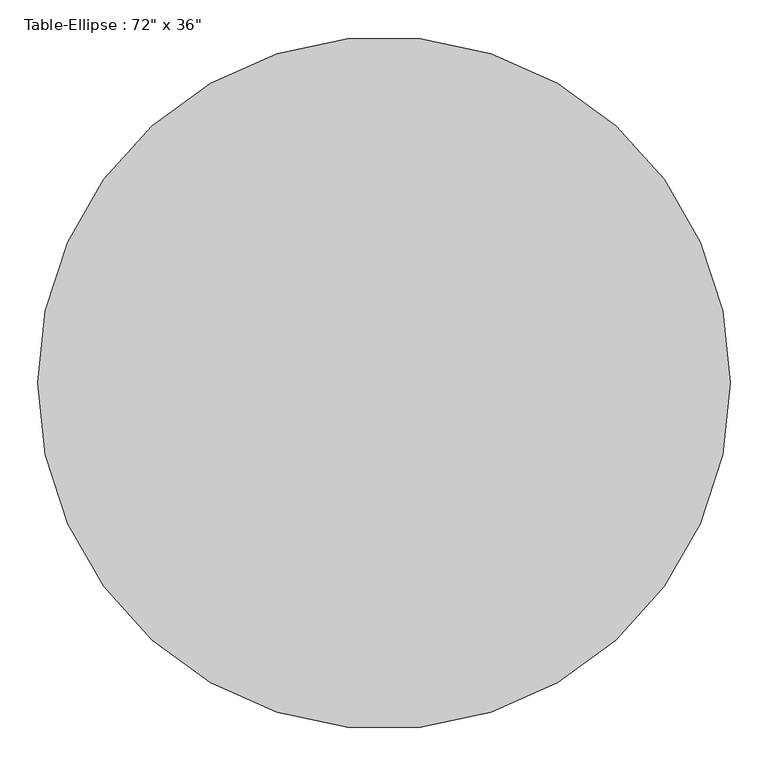
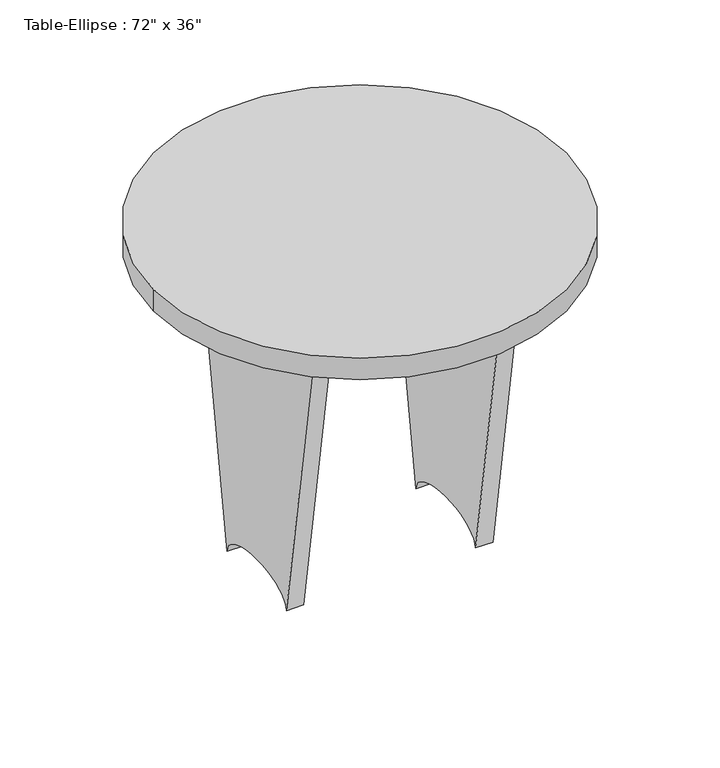
"""IFC4 building model written with IfcOpenShell, lengths in millimetres: furniture geometry."""

from ifc_helpers import new_model, si_unit, point, frame, origin, place, context, project, spatial, circle_curve, ellipse_curve, trimmed, source, transform, mapped, element, save
from ifc_brep_helpers import plane_surface, extruded_surface, advanced_brep


def furniture_4bee3317(model_context):
    return source(origin(), model_context, "Body", "AdvancedBrep", [
        advanced_brep(
        [(-190.5, 19.05, 711.2), (190.5, 19.05, 711.2), (190.5, 19.05, 474.1333333), (-190.5, 19.05, 474.1333333), (-190.5, -19.05, 711.2), (-190.5, -19.05, 474.1333333), (190.5, -19.05, 474.1333333), (190.5, -19.05, 711.2)],
        [
            (0, 1),
            (1, 2),
            (2, 3, ellipse_curve(frame((0.0, 19.05, 474.1333333), z_axis=(0.0, -1.0, 0.0), x_axis=(1.0, 0.0, 0.0)), 190.5, 101.6)),
            (3, 0),
            (4, 5),
            (5, 6, ellipse_curve(frame((0.0, -19.05, 474.1333333), z_axis=(0.0, 1.0, 0.0), x_axis=(1.0, 0.0, 0.0)), 190.5, 101.6)),
            (6, 7),
            (7, 4),
            (0, 4),
            (7, 1),
            (6, 2),
            (5, 3),
        ],
        [
            plane_surface(frame((-190.5, 19.05, 711.2), z_axis=(0.0, 1.0, 0.0), x_axis=(1.0, 0.0, 0.0))),
            plane_surface(frame((-190.5, -19.05, 711.2), z_axis=(0.0, -1.0, 0.0), x_axis=(-1.0, 0.0, 0.0))),
            plane_surface(frame((-190.5, 19.05, 711.2), z_axis=(0.0, 0.0, 1.0), x_axis=(0.0, -1.0, 0.0))),
            plane_surface(frame((190.5, 19.05, 711.2), z_axis=(1.0, 0.0, 0.0), x_axis=(0.0, -1.0, 0.0))),
            extruded_surface(trimmed(ellipse_curve(frame((0.0, -57.15, 474.1333333), z_axis=(0.0, -1.0, 0.0), x_axis=(1.0, 0.0, 0.0)), 190.5, 101.6), [point((190.5, -57.15, 474.1333333))], [point((-190.5, -57.15, 474.1333333))], True, "CARTESIAN"), (0.0, 38.099999999999994, 0.0), 38.099999999999994),
            plane_surface(frame((-190.5, 19.05, 474.1333333), z_axis=(-1.0, 0.0, 0.0), x_axis=(0.0, -1.0, 0.0))),
        ],
        [
            (0, [[1, 2, 3, 4]]),
            (1, [[5, 6, 7, 8]]),
            (2, [[-1, 9, -8, 10]]),
            (3, [[-2, -10, -7, 11]]),
            (4, [[-3, -11, -6, 12]]),
            (5, [[-4, -12, -5, -9]]),
        ],
    ),
        advanced_brep(
        [(228.6, 228.6, 711.2), (228.6, -228.6, 711.2), (228.6, -114.3, 0.0), (228.6, 114.3, 0.0), (190.5, 228.6, 711.2), (190.5, 114.3, 0.0), (190.5, -114.3, 0.0), (190.5, -228.6, 711.2)],
        [
            (0, 1),
            (1, 2),
            (2, 3, ellipse_curve(frame((228.6, 0.0, 0.0), z_axis=(-1.0, 0.0, 0.0), x_axis=(0.0, 1.0, 0.0)), 114.3, 50.8)),
            (3, 0),
            (4, 5),
            (5, 6, ellipse_curve(frame((190.5, 0.0, 0.0), z_axis=(1.0, 0.0, 0.0), x_axis=(0.0, 1.0, 0.0)), 114.3, 50.8)),
            (6, 7),
            (7, 4),
            (0, 4),
            (7, 1),
            (6, 2),
            (5, 3),
        ],
        [
            plane_surface(frame((228.6, -228.6, 711.2), z_axis=(1.0, 0.0, 0.0), x_axis=(0.0, -1.0, 0.0))),
            plane_surface(frame((190.5, -228.6, 711.2), z_axis=(-1.0, 0.0, 0.0), x_axis=(0.0, 1.0, 0.0))),
            plane_surface(frame((228.6, 228.6, 711.2), z_axis=(0.0, 0.0, 1.0), x_axis=(-1.0, 0.0, 0.0))),
            plane_surface(frame((228.6, -228.6, 711.2), z_axis=(0.0, -0.9873303712766982, -0.158678095383759), x_axis=(-1.0, 0.0, 0.0))),
            extruded_surface(trimmed(ellipse_curve(frame((152.4, 0.0, 0.0), z_axis=(-1.0, 0.0, 0.0), x_axis=(0.0, 1.0, 0.0)), 114.3, 50.8), [point((152.4, -114.3, 0.0))], [point((152.4, 114.3, 0.0))], True, "CARTESIAN"), (38.099999999999994, 0.0, 0.0), 38.099999999999994),
            plane_surface(frame((228.6, 114.3, 0.0), z_axis=(0.0, 0.9873303712767002, -0.15867809538374666), x_axis=(-1.0, 0.0, 0.0))),
        ],
        [
            (0, [[1, 2, 3, 4]]),
            (1, [[5, 6, 7, 8]]),
            (2, [[-1, 9, -8, 10]]),
            (3, [[-2, -10, -7, 11]]),
            (4, [[-3, -11, -6, 12]]),
            (5, [[-4, -12, -5, -9]]),
        ],
    ),
        advanced_brep(
        [(-190.5, 228.6, 711.2), (-190.5, -228.6, 711.2), (-190.5, -114.3, 0.0), (-190.5, 114.3, 0.0), (-228.6, 228.6, 711.2), (-228.6, 114.3, 0.0), (-228.6, -114.3, 0.0), (-228.6, -228.6, 711.2)],
        [
            (0, 1),
            (1, 2),
            (2, 3, ellipse_curve(frame((-190.5, 0.0, 0.0), z_axis=(-1.0, 0.0, 0.0), x_axis=(0.0, 1.0, 0.0)), 114.3, 50.8)),
            (3, 0),
            (4, 5),
            (5, 6, ellipse_curve(frame((-228.6, 0.0, 0.0), z_axis=(1.0, 0.0, 0.0), x_axis=(0.0, 1.0, 0.0)), 114.3, 50.8)),
            (6, 7),
            (7, 4),
            (0, 4),
            (7, 1),
            (6, 2),
            (5, 3),
        ],
        [
            plane_surface(frame((-190.5, -228.6, 711.2), z_axis=(1.0, 0.0, 0.0), x_axis=(0.0, -1.0, 0.0))),
            plane_surface(frame((-228.6, -228.6, 711.2), z_axis=(-1.0, 0.0, 0.0), x_axis=(0.0, 1.0, 0.0))),
            plane_surface(frame((-190.5, 228.6, 711.2), z_axis=(0.0, 0.0, 1.0), x_axis=(-1.0, 0.0, 0.0))),
            plane_surface(frame((-190.5, -228.6, 711.2), z_axis=(0.0, -0.9873303712766983, -0.15867809538375854), x_axis=(-1.0, 0.0, 0.0))),
            extruded_surface(trimmed(ellipse_curve(frame((-266.7, 0.0, 0.0), z_axis=(-1.0, 0.0, 0.0), x_axis=(0.0, 1.0, 0.0)), 114.3, 50.8), [point((-266.7, -114.3, 0.0))], [point((-266.7, 114.3, 0.0))], True, "CARTESIAN"), (38.099999999999994, 0.0, 0.0), 38.099999999999994),
            plane_surface(frame((-190.5, 114.3, 0.0), z_axis=(0.0, 0.9873303712766998, -0.15867809538374977), x_axis=(-1.0, 0.0, 0.0))),
        ],
        [
            (0, [[1, 2, 3, 4]]),
            (1, [[5, 6, 7, 8]]),
            (2, [[-1, 9, -8, 10]]),
            (3, [[-2, -10, -7, 11]]),
            (4, [[-3, -11, -6, 12]]),
            (5, [[-4, -12, -5, -9]]),
        ],
    ),
        advanced_brep(
        [(-457.2, 0.0, 762.0), (457.2, 0.0, 762.0), (-457.2, 0.0, 711.2), (457.2, 0.0, 711.2)],
        [
            (0, 1, circle_curve(frame((0.0, 0.0, 762.0), z_axis=(0.0, 0.0, 1.0), x_axis=(1.0, 0.0, 0.0)), 457.2)),
            (1, 0, circle_curve(frame((0.0, 0.0, 762.0), z_axis=(0.0, 0.0, 1.0), x_axis=(1.0, 0.0, 0.0)), 457.2)),
            (2, 3, ellipse_curve(frame((0.0, 0.0, 711.2), z_axis=(0.0, 0.0, -1.0), x_axis=(1.0, 0.0, 0.0)), 457.2, 457.2)),
            (3, 2, ellipse_curve(frame((0.0, 0.0, 711.2), z_axis=(0.0, 0.0, -1.0), x_axis=(1.0, 0.0, 0.0)), 457.2, 457.2)),
            (0, 2),
            (3, 1),
        ],
        [
            plane_surface(frame((457.2, 0.0, 762.0), z_axis=(0.0, 0.0, 1.0), x_axis=(0.0, 1.0, 0.0))),
            plane_surface(frame((457.2, 0.0, 711.2), z_axis=(0.0, 0.0, -1.0), x_axis=(0.0, -1.0, 0.0))),
            extruded_surface(trimmed(ellipse_curve(frame((0.0, 0.0, 660.4), z_axis=(0.0, 0.0, 1.0), x_axis=(1.0, 0.0, 0.0)), 457.2, 457.2), [point((-457.2, 0.0, 660.4))], [point((457.2, 0.0, 660.4))], True, "CARTESIAN"), (0.0, 0.0, 50.80000000000007), 50.80000000000007),
            extruded_surface(trimmed(ellipse_curve(frame((0.0, 0.0, 660.4), z_axis=(0.0, 0.0, 1.0), x_axis=(1.0, 0.0, 0.0)), 457.2, 457.2), [point((457.2, 0.0, 660.4))], [point((-457.2, 0.0, 660.4))], True, "CARTESIAN"), (0.0, 0.0, 50.80000000000007), 50.80000000000007),
        ],
        [
            (0, [[1, 2]]),
            (1, [[3, 4]]),
            (2, [[-1, 5, -4, 6]]),
            (3, [[-2, -6, -3, -5]]),
        ],
    ),
    ])


if __name__ == "__main__":
    model = new_model("IFC4")
    model_context = context("Model", 3, world=origin())
    ifc_project = project(units=[si_unit("LENGTHUNIT", "METRE", prefix="MILLI")], contexts=[model_context])
    site = spatial("IfcSite", under=ifc_project)
    building = spatial("IfcBuilding", under=site)
    placement = place(None, origin())
    furniture_shape = furniture_4bee3317(model_context)
    element("IfcFurniture", 1, ObjectType="Table-Ellipse : 72\" x 36\"", at=placement, inside=building, context=model_context, shape_type="MappedRepresentation", body=[
        mapped(furniture_shape, transform((0.0, 0.0, 0.0), x_axis=(1.0, 0.0, 0.0), y_axis=(0.0, 1.0, 0.0), z_axis=(0.0, 0.0, 1.0))),
    ])
    save(model, "model.ifc")

# Revit data of these elements
# Type "Table-Ellipse : 72\" x 36\""
#   Assembly Code = "E2020200"
#   Half Width = 1' - 6"
#   Half Length = 1' - 6"
#   Height = 2' - 6"
#   Length = 3' - 0"
#   Width = 3' - 0"
#   Base Material = Birch
#   Top Material = Laminate - Black
#   Default Elevation = 0
# Element 1 (IfcFurniture, "Table-Ellipse : 72\" x 36\"")
#   Materials on its faces: "Birch", "Laminate - Black"
# Materials
#   "Birch": class "Wood", colour RGB 224 178 126, transparency 0, Description = "Betula Alleghaniensis", Cost = 0
#   "Laminate - Black": colour RGB 0 0 0, transparency 0
